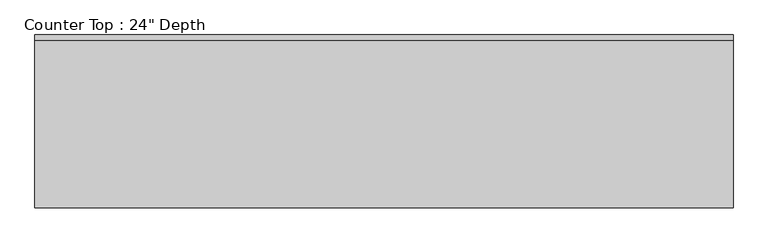
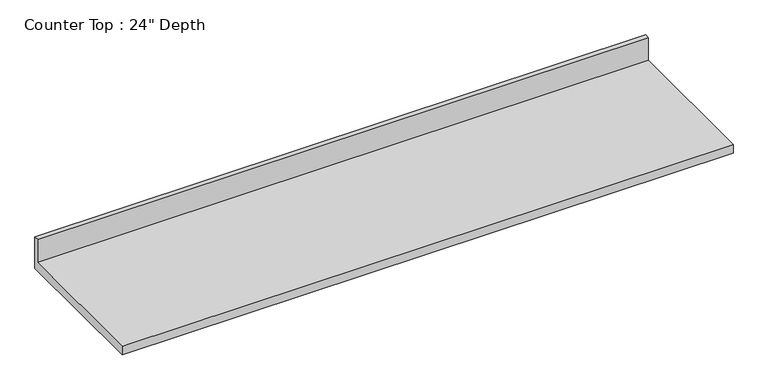
"""IFC4 building model written with IfcOpenShell, lengths in millimetres: furniture geometry."""

from ifc_helpers import new_model, si_unit, frame, origin, place, context, project, spatial, polyline, outline, extrude, source, transform, mapped, element, save


def furniture_90663022(model_context):
    return source(origin(), model_context, "Body", "SweptSolid", [
        extrude(outline(polyline([(0.0, 1016.0), (0.0, 876.3), (-635.0, 876.3), (-635.0, 914.4), (-19.05, 914.4), (-19.05, 1016.0), (0.0, 1016.0)])), frame((-1200.4622951, 0.0, 0.0), z_axis=(1.0, 0.0, 0.0), x_axis=(0.0, 1.0, 0.0)), (0.0, 0.0, 1.0), 2565.4),
    ])


if __name__ == "__main__":
    model = new_model("IFC4")
    model_context = context("Model", 3, world=origin())
    ifc_project = project(units=[si_unit("LENGTHUNIT", "METRE", prefix="MILLI")], contexts=[model_context])
    site = spatial("IfcSite", under=ifc_project)
    building = spatial("IfcBuilding", under=site)
    placement = place(None, origin())
    furniture_shape = furniture_90663022(model_context)
    element("IfcFurniture", 1, ObjectType="Counter Top : 24\" Depth", at=placement, inside=building, context=model_context, shape_type="MappedRepresentation", body=[
        mapped(furniture_shape, transform((0.0, 0.0, 0.0), x_axis=(1.0, 0.0, 0.0), y_axis=(0.0, 1.0, 0.0), z_axis=(0.0, 0.0, 1.0))),
    ])
    save(model, "model.ifc")

# Revit data of these elements
# Type "Counter Top : 24\" Depth"
#   Assembly Code = "C1030400"
#   Counter Thickness = 0' - 1 1/2"
#   Depth = 2' - 1"
#   Height = 3' - 0"
#   Length [instance default] = 8' - 0"
#   Counter Top Material = none
#   Default Elevation = 0
# Element 1 (IfcFurniture, "Counter Top : 24\" Depth")
#   Length = 8' - 5"
#   Materials on its faces: "Counter Top"
# Materials
#   "Counter Top": class "Wood", colour RGB 226 177 128, transparency 0
